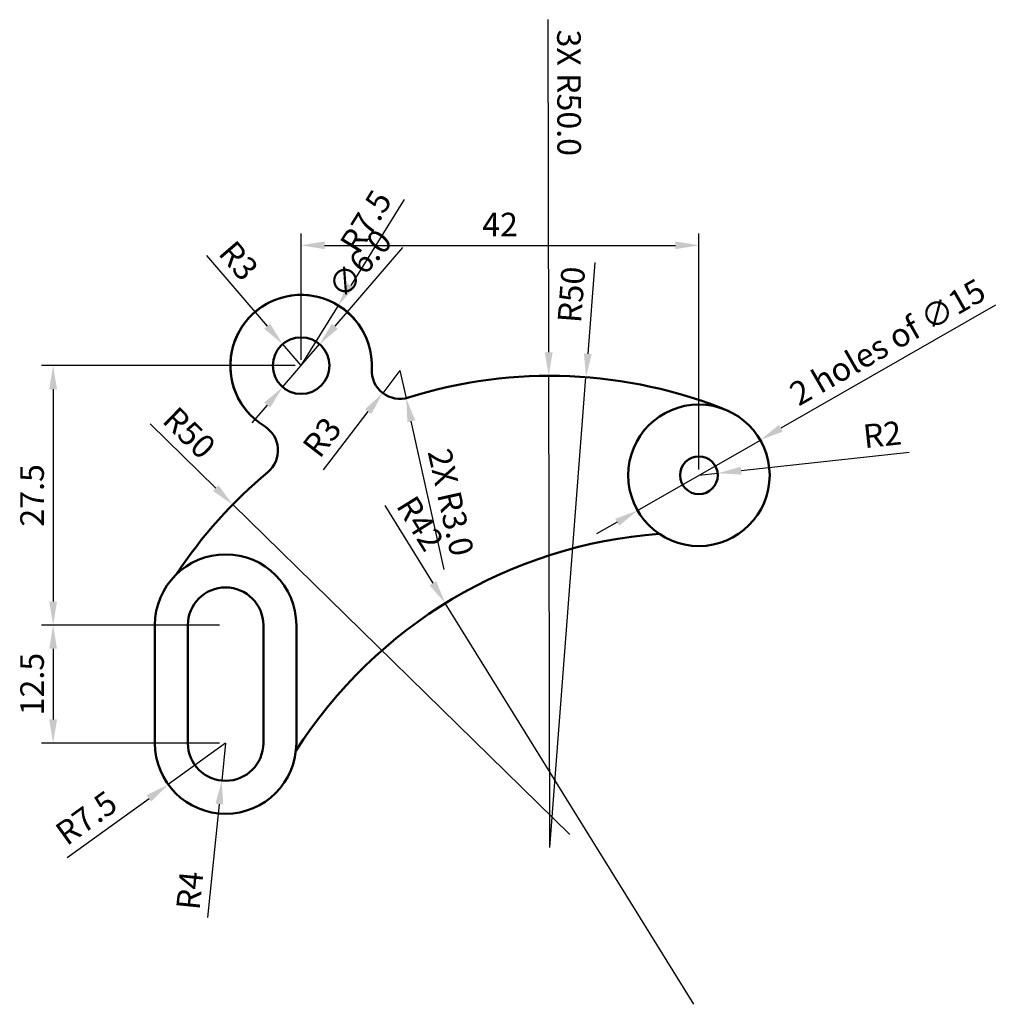
# Model space of a CAD drawing. Units: millimetres. Extents: x 3006 to 3110, y 1787 to 1891.
import ezdxf

# ---------------------------------------------------------------- set-up
doc = ezdxf.new("R2010")
doc.units = ezdxf.units.MM
doc.layers.add('M-DIMS', color=2, linetype='Continuous', lineweight=25)
doc.layers.add('M-OUTL', color=7, linetype='Continuous', lineweight=50)
doc.styles.get("Standard").update_dxf_attribs({"font": 'arial.ttf'})
doc.dimstyles.new('ISO-25', dxfattribs={"dimtxt": 2.5, "dimasz": 2.5, "dimexe": 1.25, "dimexo": 0.625, "dimtad": 1, "dimdec": 1, "dimdsep": 46, "dimtxsty": 'Standard', "dimcen": 2.5, "dimadec": 0, "dimazin": 0, "dimtfac": 1, "dimtdec": 1, "dimtmove": 0, "dimatfit": 3, "dimfxl": 1, "dimarcsym": 0})

# ---------------------------------------------------------------- blocks, each defined once
blk = doc.blocks.new('*D1')
at = {"layer": 'Defpoints', "color": 0, "transparency": 16777216}
for p in [(3028.8, 1839.91), (3064.53, 1804.94)]:
    blk.add_point(p, dxfattribs=at)
at = {"layer": 'M-DIMS', "color": 0, "lineweight": -2, "transparency": 16777216}
for p, q in [((3020.07, 1848.46), (3027.01, 1841.66)), ((3064.53, 1804.94), (3028.8, 1839.91))]:
    blk.add_line(p, q, dxfattribs=at)
at = {"layer": 'M-DIMS', "color": 0, "transparency": 16777216}
blk.add_solid([(3027.3, 1841.96), (3026.72, 1841.36), (3028.8, 1839.91)], dxfattribs=at)
at = {"layer": 'M-DIMS', "color": 0, "transparency": 16777216, "insert": (3023.98, 1847.29), "char_height": 2.5, "attachment_point": 5, "rotation": 315.6135}
blk.add_mtext('R50', dxfattribs=at)
blk = doc.blocks.new('*D2')
at = {"layer": 'Defpoints', "color": 0, "transparency": 16777216}
for p in [(3051.34, 1829.45), (3077.67, 1786.95)]:
    blk.add_point(p, dxfattribs=at)
at = {"layer": 'M-DIMS', "color": 0, "lineweight": -2, "transparency": 16777216}
for p, q in [((3044.91, 1839.82), (3050.02, 1831.58)), ((3077.67, 1786.95), (3051.34, 1829.45))]:
    blk.add_line(p, q, dxfattribs=at)
at = {"layer": 'M-DIMS', "color": 0, "transparency": 16777216}
blk.add_solid([(3050.37, 1831.8), (3049.67, 1831.36), (3051.34, 1829.45)], dxfattribs=at)
at = {"layer": 'M-DIMS', "color": 0, "transparency": 16777216, "insert": (3048.41, 1837.75), "char_height": 2.5, "attachment_point": 5, "rotation": 301.7845}
blk.add_mtext('R42', dxfattribs=at)
blk = doc.blocks.new('*D3')
at = {"layer": 'Defpoints', "color": 0, "transparency": 16777216}
for p in [(3078.22, 1843.02), (3080.21, 1843.24)]:
    blk.add_point(p, dxfattribs=at)
at = {"layer": 'M-DIMS', "color": 0, "lineweight": -2, "transparency": 16777216}
for p, q in [((3100.51, 1845.43), (3082.7, 1843.5)), ((3078.22, 1843.02), (3080.21, 1843.24))]:
    blk.add_line(p, q, dxfattribs=at)
at = {"layer": 'M-DIMS', "color": 0, "transparency": 16777216}
blk.add_solid([(3082.65, 1843.92), (3082.74, 1843.09), (3080.21, 1843.24)], dxfattribs=at)
at = {"layer": 'M-DIMS', "color": 0, "transparency": 16777216, "insert": (3097.69, 1847.02), "char_height": 2.5, "attachment_point": 5, "rotation": 6.1632}
blk.add_mtext('R2', dxfattribs=at)
blk = doc.blocks.new('*D4')
at = {"layer": 'Defpoints', "color": 0, "transparency": 16777216}
for p in [(3046.53, 1854.12), (3044.7, 1851.74)]:
    blk.add_point(p, dxfattribs=at)
at = {"layer": 'M-DIMS', "color": 0, "lineweight": -2, "transparency": 16777216}
for p, q in [((3046.53, 1854.12), (3044.7, 1851.74)), ((3038.42, 1843.61), (3043.17, 1849.77))]:
    blk.add_line(p, q, dxfattribs=at)
at = {"layer": 'M-DIMS', "color": 0, "transparency": 16777216}
blk.add_solid([(3042.84, 1850.02), (3043.5, 1849.51), (3044.7, 1851.74)], dxfattribs=at)
at = {"layer": 'M-DIMS', "color": 0, "transparency": 16777216, "insert": (3038.52, 1846.86), "char_height": 2.5, "attachment_point": 5, "rotation": 52.3146}
blk.add_mtext('R3', dxfattribs=at)
blk = doc.blocks.new('*D5')
at = {"layer": 'Defpoints', "color": 0, "transparency": 16777216}
for p in [(3066.25, 1853.41), (3062.43, 1803.56)]:
    blk.add_point(p, dxfattribs=at)
at = {"layer": 'M-DIMS', "color": 0, "lineweight": -2, "transparency": 16777216}
for p, q in [((3067.19, 1865.59), (3066.44, 1855.9)), ((3062.43, 1803.56), (3066.25, 1853.41))]:
    blk.add_line(p, q, dxfattribs=at)
at = {"layer": 'M-DIMS', "color": 0, "transparency": 16777216}
blk.add_solid([(3066.03, 1855.94), (3066.86, 1855.87), (3066.25, 1853.41)], dxfattribs=at)
at = {"layer": 'M-DIMS', "color": 0, "transparency": 16777216, "insert": (3065.02, 1862.14), "char_height": 2.5, "attachment_point": 5, "rotation": 85.6107}
blk.add_mtext('R50', dxfattribs=at)
blk = doc.blocks.new('*D6')
at = {"layer": 'Defpoints', "color": 0, "transparency": 16777216}
for p in [(3034.1, 1856.91), (3036.05, 1854.64)]:
    blk.add_point(p, dxfattribs=at)
at = {"layer": 'M-DIMS', "color": 0, "lineweight": -2, "transparency": 16777216}
for p, q in [((3026.02, 1866.33), (3032.47, 1858.81)), ((3036.05, 1854.64), (3034.1, 1856.91))]:
    blk.add_line(p, q, dxfattribs=at)
at = {"layer": 'M-DIMS', "color": 0, "transparency": 16777216}
blk.add_solid([(3032.78, 1859.08), (3032.15, 1858.54), (3034.1, 1856.91)], dxfattribs=at)
at = {"layer": 'M-DIMS', "color": 0, "transparency": 16777216, "insert": (3029.19, 1865.56), "char_height": 2.5, "attachment_point": 5, "rotation": 310.5946}
blk.add_mtext('R3', dxfattribs=at)
blk = doc.blocks.new('*D7')
at = {"layer": 'Defpoints', "color": 0, "transparency": 16777216}
for p in [(3028.05, 1814.64), (3027.64, 1810.66)]:
    blk.add_point(p, dxfattribs=at)
at = {"layer": 'M-DIMS', "color": 0, "lineweight": -2, "transparency": 16777216}
for p, q in [((3028.05, 1814.64), (3027.64, 1810.66)), ((3026.17, 1796.17), (3027.39, 1808.17))]:
    blk.add_line(p, q, dxfattribs=at)
at = {"layer": 'M-DIMS', "color": 0, "transparency": 16777216}
blk.add_solid([(3026.98, 1808.21), (3027.8, 1808.13), (3027.64, 1810.66)], dxfattribs=at)
at = {"layer": 'M-DIMS', "color": 0, "transparency": 16777216, "insert": (3024.57, 1798.98), "char_height": 2.5, "attachment_point": 5, "rotation": 84.1962}
blk.add_mtext('R4', dxfattribs=at)
blk = doc.blocks.new('*D8')
at = {"layer": 'Defpoints', "color": 0, "transparency": 16777216}
for p in [(3028.05, 1814.64), (3021.97, 1810.25)]:
    blk.add_point(p, dxfattribs=at)
at = {"layer": 'M-DIMS', "color": 0, "lineweight": -2, "transparency": 16777216}
for p, q in [((3028.05, 1814.64), (3021.97, 1810.25)), ((3011.25, 1802.51), (3019.94, 1808.78))]:
    blk.add_line(p, q, dxfattribs=at)
at = {"layer": 'M-DIMS', "color": 0, "transparency": 16777216}
blk.add_solid([(3019.69, 1809.12), (3020.18, 1808.45), (3021.97, 1810.25)], dxfattribs=at)
at = {"layer": 'M-DIMS', "color": 0, "transparency": 16777216, "insert": (3013.47, 1806.45), "char_height": 2.5, "attachment_point": 5, "rotation": 35.8183}
blk.add_mtext('R7.5', dxfattribs=at)
blk = doc.blocks.new('*D9')
at = {"layer": 'Defpoints', "color": 0, "transparency": 16777216}
for p in [(3084.73, 1846.76), (3071.72, 1839.29)]:
    blk.add_point(p, dxfattribs=at)
at = {"layer": 'M-DIMS', "color": 0, "lineweight": -2, "transparency": 16777216}
for p, q in [((3109.64, 1861.06), (3086.9, 1848)), ((3071.72, 1839.29), (3084.73, 1846.76)), ((3069.55, 1838.04), (3067.38, 1836.8))]:
    blk.add_line(p, q, dxfattribs=at)
at = {"layer": 'M-DIMS', "color": 0, "transparency": 16777216}
for points in [[(3086.69, 1848.36), (3087.1, 1847.64), (3084.73, 1846.76)], [(3069.35, 1838.4), (3069.76, 1837.68), (3071.72, 1839.29)]]:
    blk.add_solid(points, dxfattribs=at)
at = {"layer": 'M-DIMS', "color": 0, "transparency": 16777216, "insert": (3098.37, 1856.86), "char_height": 2.5, "attachment_point": 5, "rotation": 29.8709}
blk.add_mtext('2 holes of ∅15', dxfattribs=at)
blk = doc.blocks.new('*D10')
at = {"layer": 'Defpoints', "color": 0, "transparency": 16777216}
for p in [(3078.22, 1867.39), (3036.05, 1854.64), (3078.22, 1843.02)]:
    blk.add_point(p, dxfattribs=at)
at = {"layer": 'M-DIMS', "color": 0, "lineweight": -2, "transparency": 16777216}
for p, q in [((3036.05, 1855.26), (3036.05, 1868.64)), ((3078.22, 1843.65), (3078.22, 1868.64)), ((3038.55, 1867.39), (3075.72, 1867.39))]:
    blk.add_line(p, q, dxfattribs=at)
at = {"layer": 'M-DIMS', "color": 0, "transparency": 16777216}
for points in [[(3038.55, 1867.81), (3038.55, 1866.98), (3036.05, 1867.39)], [(3075.72, 1867.81), (3075.72, 1866.98), (3078.22, 1867.39)]]:
    blk.add_solid(points, dxfattribs=at)
at = {"layer": 'M-DIMS', "color": 0, "transparency": 16777216, "insert": (3057.14, 1869.27), "char_height": 2.5, "attachment_point": 5}
blk.add_mtext('42', dxfattribs=at)
blk = doc.blocks.new('*D11')
at = {"layer": 'Defpoints', "color": 0, "transparency": 16777216}
for p in [(3036.05, 1854.64), (3009.77, 1827.14), (3028.05, 1827.14)]:
    blk.add_point(p, dxfattribs=at)
at = {"layer": 'M-DIMS', "color": 0, "lineweight": -2, "transparency": 16777216}
for p, q in [((3035.42, 1854.64), (3008.52, 1854.64)), ((3009.77, 1852.14), (3009.77, 1829.64)), ((3027.42, 1827.14), (3008.52, 1827.14))]:
    blk.add_line(p, q, dxfattribs=at)
at = {"layer": 'M-DIMS', "color": 0, "transparency": 16777216}
for points in [[(3009.35, 1852.14), (3010.18, 1852.14), (3009.77, 1854.64)], [(3009.35, 1829.64), (3010.18, 1829.64), (3009.77, 1827.14)]]:
    blk.add_solid(points, dxfattribs=at)
at = {"layer": 'M-DIMS', "color": 0, "transparency": 16777216, "insert": (3007.86, 1840.89), "char_height": 2.5, "attachment_point": 5, "rotation": 90}
blk.add_mtext('27.5', dxfattribs=at)
blk = doc.blocks.new('*D12')
at = {"layer": 'Defpoints', "color": 0, "transparency": 16777216}
for p in [(3028.05, 1827.14), (3009.77, 1814.64), (3028.05, 1814.64)]:
    blk.add_point(p, dxfattribs=at)
at = {"layer": 'M-DIMS', "color": 0, "lineweight": -2, "transparency": 16777216}
for p, q in [((3027.42, 1827.14), (3008.52, 1827.14)), ((3009.77, 1824.64), (3009.77, 1817.14)), ((3027.42, 1814.64), (3008.52, 1814.64))]:
    blk.add_line(p, q, dxfattribs=at)
at = {"layer": 'M-DIMS', "color": 0, "transparency": 16777216}
for points in [[(3009.35, 1824.64), (3010.18, 1824.64), (3009.77, 1827.14)], [(3009.35, 1817.14), (3010.18, 1817.14), (3009.77, 1814.64)]]:
    blk.add_solid(points, dxfattribs=at)
at = {"layer": 'M-DIMS', "color": 0, "transparency": 16777216, "insert": (3007.86, 1820.89), "char_height": 2.5, "attachment_point": 5, "rotation": 90}
blk.add_mtext('12.5', dxfattribs=at)
blk = doc.blocks.new('*D13')
at = {"layer": 'Defpoints', "color": 0, "transparency": 16777216}
for p in [(3038, 1856.91), (3034.09, 1852.36)]:
    blk.add_point(p, dxfattribs=at)
at = {"layer": 'M-DIMS', "color": 0, "lineweight": -2, "transparency": 16777216}
for p, q in [((3046.8, 1867.16), (3039.63, 1858.81)), ((3034.09, 1852.36), (3038, 1856.91)), ((3032.46, 1850.46), (3030.84, 1848.57))]:
    blk.add_line(p, q, dxfattribs=at)
at = {"layer": 'M-DIMS', "color": 0, "transparency": 16777216}
for points in [[(3039.31, 1859.08), (3039.95, 1858.54), (3038, 1856.91)], [(3032.15, 1850.73), (3032.78, 1850.19), (3034.09, 1852.36)]]:
    blk.add_solid(points, dxfattribs=at)
at = {"layer": 'M-DIMS', "color": 0, "transparency": 16777216, "insert": (3042.53, 1865.22), "char_height": 2.5, "attachment_point": 5, "rotation": 49.3551}
blk.add_mtext('∅6.0', dxfattribs=at)
blk = doc.blocks.new('*D14')
at = {"layer": 'Defpoints', "color": 0, "transparency": 16777216}
for p in [(3040, 1861.01), (3036.05, 1854.64)]:
    blk.add_point(p, dxfattribs=at)
at = {"layer": 'M-DIMS', "color": 0, "lineweight": -2, "transparency": 16777216}
for p, q in [((3046.96, 1872.24), (3041.32, 1863.13)), ((3036.05, 1854.64), (3040, 1861.01))]:
    blk.add_line(p, q, dxfattribs=at)
at = {"layer": 'M-DIMS', "color": 0, "transparency": 16777216}
blk.add_solid([(3040.96, 1863.35), (3041.67, 1862.91), (3040, 1861.01)], dxfattribs=at)
at = {"layer": 'M-DIMS', "color": 0, "transparency": 16777216, "insert": (3043.19, 1869.75), "char_height": 2.5, "attachment_point": 5, "rotation": 58.1981}
blk.add_mtext('R7.5', dxfattribs=at)
blk = doc.blocks.new('*D15')
at = {"layer": 'Defpoints', "color": 0, "transparency": 16777216}
for p in [(3046.53, 1854.12), (3047.19, 1851.19)]:
    blk.add_point(p, dxfattribs=at)
at = {"layer": 'M-DIMS', "color": 0, "lineweight": -2, "transparency": 16777216}
for p, q in [((3046.53, 1854.12), (3047.19, 1851.19)), ((3051.23, 1833.04), (3047.73, 1848.75))]:
    blk.add_line(p, q, dxfattribs=at)
at = {"layer": 'M-DIMS', "color": 0, "transparency": 16777216}
blk.add_solid([(3048.14, 1848.84), (3047.32, 1848.66), (3047.19, 1851.19)], dxfattribs=at)
at = {"layer": 'M-DIMS', "color": 0, "transparency": 16777216, "insert": (3051.61, 1840.09), "char_height": 2.5, "attachment_point": 5, "rotation": 282.5611}
blk.add_mtext('2X R3.0', dxfattribs=at)
blk = doc.blocks.new('*D16')
at = {"layer": 'Defpoints', "color": 0, "transparency": 16777216}
for p in [(3062.3, 1853.56), (3062.43, 1803.56)]:
    blk.add_point(p, dxfattribs=at)
at = {"layer": 'M-DIMS', "color": 0, "lineweight": -2, "transparency": 16777216}
for p, q in [((3062.2, 1891.31), (3062.29, 1856.06)), ((3062.43, 1803.56), (3062.3, 1853.56))]:
    blk.add_line(p, q, dxfattribs=at)
at = {"layer": 'M-DIMS', "color": 0, "transparency": 16777216}
blk.add_solid([(3062.71, 1856.06), (3061.88, 1856.06), (3062.3, 1853.56)], dxfattribs=at)
at = {"layer": 'M-DIMS', "color": 0, "transparency": 16777216, "insert": (3064.13, 1883.56), "char_height": 2.5, "attachment_point": 5, "rotation": 270.1449}
blk.add_mtext('3X R50.0', dxfattribs=at)

msp = doc.modelspace()

# ---------------------------------------------------------------- linework, layer by layer
at = {"layer": 'M-OUTL'}
for p, q in [((3020.55, 1827.14), (3020.55, 1814.64)), ((3024.05, 1827.14), (3024.05, 1814.64)), ((3032.05, 1827.14), (3032.05, 1814.64)), ((3035.55, 1827.14), (3035.55, 1814.64))]:
    msp.add_line(p, q, dxfattribs=at)
for centre, radius in [((3036.05, 1854.64), 3), ((3078.22, 1843.02), 7.5), ((3078.22, 1843.02), 2)]:
    msp.add_circle(centre, radius, dxfattribs=at)
for centre, radius, start, end in [((3036.05, 1854.64), 7.5, 17.8872, 229.7486), ((3036.05, 1854.64), 7.5, 357.1812, 238.7752), ((3046.53, 1854.12), 3, 177.1812, 287.4481), ((3062.43, 1803.56), 50, 67.7256, 107.4481), ((3030.6, 1845.66), 3, 309.7993, 58.7752), ((3064.53, 1804.94), 50, 129.7993, 146.5211), ((3077.67, 1786.95), 50, 94.2022, 147.5036), ((3028.05, 1827.14), 7.5, 0, 180), ((3028.05, 1827.14), 4, 0, 180), ((3028.05, 1814.64), 7.5, 180, 0), ((3028.05, 1814.64), 4, 180, 0)]:
    msp.add_arc(centre, radius, start, end, dxfattribs=at)

# ---------------------------------------------------------------- dimensions: what is measured, and where the dimension line sits
at = {"layer": 'M-DIMS'}
dim = msp.add_radius_dim(center=(3062.43, 1803.56), mpoint=(3062.3, 1853.56), text='3X <>', dimstyle='ISO-25', override={"dimdec": 1, "dimlfac": 1, "dimrnd": 0, "dimzin": 0, "dimdsep": 46, "dimlunit": 2}, dxfattribs=at)
dim.commit()
dim.dimension.update_dxf_attribs({"geometry": '*D16', "text_midpoint": (3062.22, 1883.56), "dimtype": 164})
for center, mpoint, override, picture, middle in [((3036.05, 1854.64), (3040, 1861.01), {"dimdec": 1, "dimlfac": 1, "dimrnd": 0, "dimzin": 0, "dimdsep": 46, "dimlunit": 2}, '*D14', (3043.19, 1869.75)), ((3062.43, 1803.56), (3066.25, 1853.41), {"dimclrd": 0, "dimclre": 0, "dimclrt": 0}, '*D5', (3065.02, 1862.14)), ((3046.53, 1854.12), (3044.7, 1851.74), {"dimclrd": 0, "dimclre": 0, "dimclrt": 0}, '*D4', (3038.52, 1846.86)), ((3064.53, 1804.94), (3028.8, 1839.91), {"dimclrd": 0, "dimclre": 0, "dimclrt": 0}, '*D1', (3023.98, 1847.29)), ((3028.05, 1814.64), (3021.97, 1810.25), {"dimclrd": 0, "dimclre": 0, "dimclrt": 0}, '*D8', (3013.47, 1806.45))]:
    dim = msp.add_radius_dim(center=center, mpoint=mpoint, dimstyle='ISO-25', override=override, dxfattribs=at)
    dim.commit()
    dim.dimension.update_dxf_attribs({"geometry": picture, "text_midpoint": middle})
dim = msp.add_linear_dim(base=(3078.22, 1867.39), p1=(3036.05, 1854.64), p2=(3078.22, 1843.02), text='42', dimstyle='ISO-25', override={"dimclrd": 0, "dimclre": 0, "dimclrt": 0}, dxfattribs=at)
dim.commit()
dim.dimension.update_dxf_attribs({"geometry": '*D10', "text_midpoint": (3057.14, 1869.27)})
dim = msp.add_diameter_dim_2p(p1=(3034.09, 1852.36), p2=(3038, 1856.91), dimstyle='ISO-25', override={"dimdec": 1, "dimlfac": 1, "dimrnd": 0, "dimzin": 0, "dimdsep": 46, "dimlunit": 2}, dxfattribs=at)
dim.commit()
dim.dimension.update_dxf_attribs({"geometry": '*D13', "text_midpoint": (3044.03, 1863.93)})
for center, mpoint, picture, middle in [((3036.05, 1854.64), (3034.1, 1856.91), '*D6', (3027.74, 1864.33)), ((3078.22, 1843.02), (3080.21, 1843.24), '*D3', (3097.89, 1845.15)), ((3028.05, 1814.64), (3027.64, 1810.66), '*D7', (3026.44, 1798.79))]:
    dim = msp.add_radius_dim(center=center, mpoint=mpoint, dimstyle='ISO-25', override={"dimclrd": 0, "dimclre": 0, "dimclrt": 0}, dxfattribs=at)
    dim.commit()
    dim.dimension.update_dxf_attribs({"geometry": picture, "text_midpoint": middle, "dimtype": 164})
dim = msp.add_diameter_dim_2p(p1=(3071.72, 1839.29), p2=(3084.73, 1846.76), text='2 holes of <>', dimstyle='ISO-25', override={"dimclrd": 0, "dimclre": 0, "dimclrt": 0}, dxfattribs=at)
dim.commit()
dim.dimension.update_dxf_attribs({"geometry": '*D9', "text_midpoint": (3098.37, 1856.86)})
for base, p1, p2, picture, middle in [((3009.77, 1827.14), (3036.05, 1854.64), (3028.05, 1827.14), '*D11', (3007.86, 1840.89)), ((3009.77, 1814.64), (3028.05, 1827.14), (3028.05, 1814.64), '*D12', (3007.86, 1820.89))]:
    dim = msp.add_linear_dim(base=base, p1=p1, p2=p2, angle=90, dimstyle='ISO-25', override={"dimclrd": 0, "dimclre": 0, "dimclrt": 0}, dxfattribs=at)
    dim.commit()
    dim.dimension.update_dxf_attribs({"geometry": picture, "text_midpoint": middle})
for center, mpoint, text, override, picture, middle in [((3046.53, 1854.12), (3047.19, 1851.19), '2X <>', {"dimdec": 1, "dimlfac": 1, "dimrnd": 0, "dimzin": 0, "dimdsep": 46, "dimlunit": 2}, '*D15', (3051.61, 1840.09)), ((3077.67, 1786.95), (3051.34, 1829.45), 'R42', {"dimclrd": 0, "dimclre": 0, "dimclrt": 0}, '*D2', (3048.41, 1837.75))]:
    dim = msp.add_radius_dim(center=center, mpoint=mpoint, text=text, dimstyle='ISO-25', override=override, dxfattribs=at)
    dim.commit()
    dim.dimension.update_dxf_attribs({"geometry": picture, "text_midpoint": middle})

doc.saveas('drawing.dxf')
